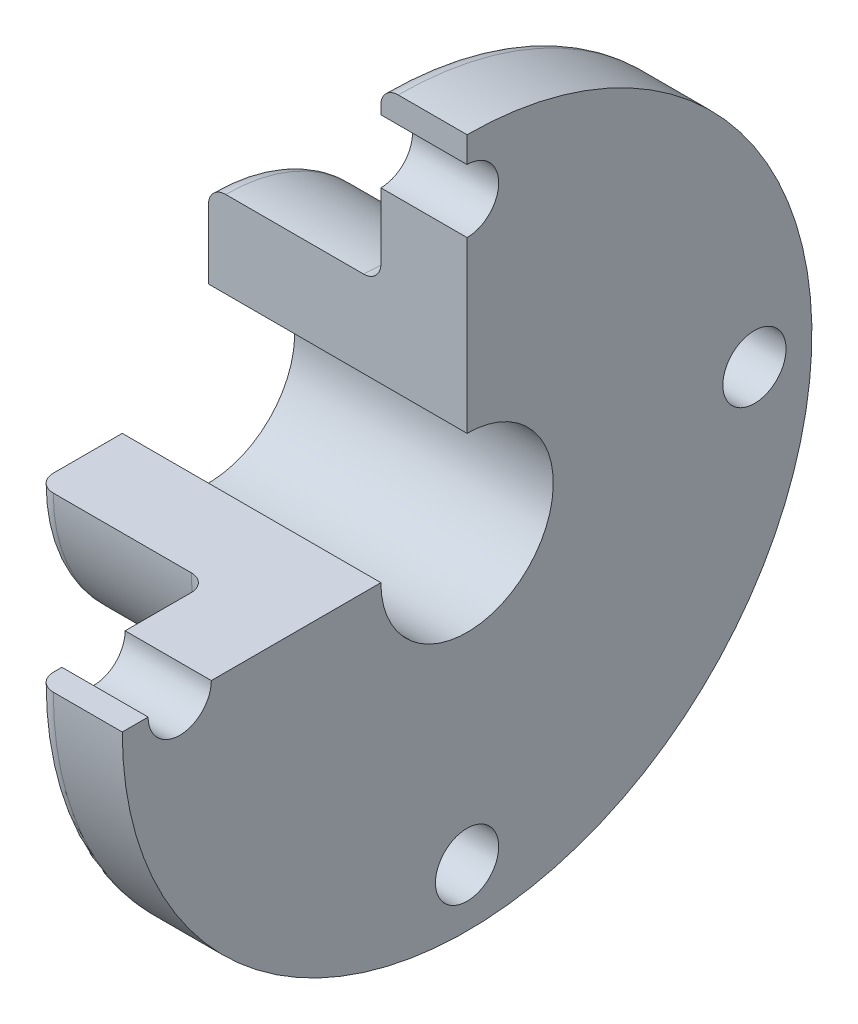
ISO-10303-21;
HEADER;
FILE_DESCRIPTION(('STEP AP214'),'2;1');
FILE_NAME('part.step','',(''),(''),'','','');
FILE_SCHEMA(('AUTOMOTIVE_DESIGN { 1 0 10303 214 1 1 1 1 }'));
ENDSEC;
DATA;
#1=APPLICATION_CONTEXT('core data for automotive mechanical design processes');
#2=APPLICATION_PROTOCOL_DEFINITION('international standard','automotive_design',2000,#1);
#3=PRODUCT_CONTEXT('',#1,'mechanical');
#4=PRODUCT('Part','Part','',(#3));
#5=PRODUCT_RELATED_PRODUCT_CATEGORY('part','',(#4));
#6=PRODUCT_DEFINITION_FORMATION('','',#4);
#7=PRODUCT_DEFINITION_CONTEXT('part definition',#1,'design');
#8=PRODUCT_DEFINITION('design','',#6,#7);
#9=PRODUCT_DEFINITION_SHAPE('','',#8);
#10=(LENGTH_UNIT() NAMED_UNIT(*) SI_UNIT(.MILLI.,.METRE.));
#11=(NAMED_UNIT(*) PLANE_ANGLE_UNIT() SI_UNIT($,.RADIAN.));
#12=(NAMED_UNIT(*) SI_UNIT($,.STERADIAN.) SOLID_ANGLE_UNIT());
#13=UNCERTAINTY_MEASURE_WITH_UNIT(LENGTH_MEASURE(1.E-05),#10,'distance_accuracy_value','');
#14=(GEOMETRIC_REPRESENTATION_CONTEXT(3) GLOBAL_UNCERTAINTY_ASSIGNED_CONTEXT((#13)) GLOBAL_UNIT_ASSIGNED_CONTEXT((#10,
#11,#12)) REPRESENTATION_CONTEXT('',''));
#15=CARTESIAN_POINT('',(0.,0.,0.));
#16=DIRECTION('',(0.,0.,1.));
#17=DIRECTION('',(1.,0.,0.));
#18=AXIS2_PLACEMENT_3D('',#15,#16,#17);
#19=CARTESIAN_POINT('',(17.9203539823009,0.,0.));
#20=DIRECTION('',(1.,0.,0.));
#21=DIRECTION('',(0.,0.,-1.));
#22=AXIS2_PLACEMENT_3D('',#19,#20,#21);
#23=PLANE('',#22);
#24=DIRECTION('',(0.,0.,1.));
#25=VECTOR('',#24,1.);
#26=CARTESIAN_POINT('',(17.9203539823009,0.,0.));
#27=LINE('',#26,#25);
#28=CARTESIAN_POINT('',(17.9203539823009,0.,55.5));
#29=VERTEX_POINT('',#28);
#30=CARTESIAN_POINT('',(17.9203539823009,0.,60.));
#31=VERTEX_POINT('',#30);
#32=EDGE_CURVE('E267',#29,#31,#27,.T.);
#33=ORIENTED_EDGE('',*,*,#32,.T.);
#34=CARTESIAN_POINT('',(17.9203539823009,0.,0.));
#35=DIRECTION('',(-1.,0.,0.));
#36=DIRECTION('',(0.,0.,1.));
#37=AXIS2_PLACEMENT_3D('',#34,#35,#36);
#38=CIRCLE('',#37,60.);
#39=CARTESIAN_POINT('',(17.9203539823009,60.,0.));
#40=VERTEX_POINT('',#39);
#41=EDGE_CURVE('E162',#40,#31,#38,.T.);
#42=ORIENTED_EDGE('',*,*,#41,.F.);
#43=DIRECTION('',(0.,-1.,0.));
#44=VECTOR('',#43,1.);
#45=CARTESIAN_POINT('',(17.9203539823009,77.9574634988186,0.));
#46=LINE('',#45,#44);
#47=CARTESIAN_POINT('',(17.9203539823009,55.5,0.));
#48=VERTEX_POINT('',#47);
#49=EDGE_CURVE('E272',#40,#48,#46,.T.);
#50=ORIENTED_EDGE('',*,*,#49,.T.);
#51=CARTESIAN_POINT('',(17.9203539823009,50.,0.));
#52=DIRECTION('',(-1.,0.,0.));
#53=DIRECTION('',(0.,0.,1.));
#54=AXIS2_PLACEMENT_3D('',#51,#52,#53);
#55=CIRCLE('',#54,5.5);
#56=CARTESIAN_POINT('',(17.9203539823009,44.5,0.));
#57=VERTEX_POINT('',#56);
#58=EDGE_CURVE('E229',#48,#57,#55,.T.);
#59=ORIENTED_EDGE('',*,*,#58,.T.);
#60=CARTESIAN_POINT('',(17.9203539823009,15.,0.));
#61=VERTEX_POINT('',#60);
#62=EDGE_CURVE('E270',#57,#61,#46,.T.);
#63=ORIENTED_EDGE('',*,*,#62,.T.);
#64=CARTESIAN_POINT('',(17.9203539823009,0.,0.));
#65=DIRECTION('',(-1.,0.,0.));
#66=DIRECTION('',(0.,0.,1.));
#67=AXIS2_PLACEMENT_3D('',#64,#65,#66);
#68=CIRCLE('',#67,15.);
#69=CARTESIAN_POINT('',(17.9203539823009,0.,15.));
#70=VERTEX_POINT('',#69);
#71=EDGE_CURVE('E231',#61,#70,#68,.T.);
#72=ORIENTED_EDGE('',*,*,#71,.T.);
#73=CARTESIAN_POINT('',(17.9203539823009,0.,44.5));
#74=VERTEX_POINT('',#73);
#75=EDGE_CURVE('E198',#70,#74,#27,.T.);
#76=ORIENTED_EDGE('',*,*,#75,.T.);
#77=CARTESIAN_POINT('',(17.9203539823009,-1.74574066942157E-13,50.));
#78=DIRECTION('',(-1.,0.,0.));
#79=DIRECTION('',(0.,0.,1.));
#80=AXIS2_PLACEMENT_3D('',#77,#78,#79);
#81=CIRCLE('',#80,5.5);
#82=EDGE_CURVE('E230',#74,#29,#81,.T.);
#83=ORIENTED_EDGE('',*,*,#82,.T.);
#84=EDGE_LOOP('',(#33,#42,#50,#59,#63,#72,#76,#83));
#85=FACE_BOUND('',#84,.T.);
#86=CARTESIAN_POINT('',(17.9203539823009,5.2372220082647E-13,-50.));
#87=DIRECTION('',(-1.,0.,0.));
#88=DIRECTION('',(0.,0.,1.));
#89=AXIS2_PLACEMENT_3D('',#86,#87,#88);
#90=CIRCLE('',#89,5.5);
#91=CARTESIAN_POINT('',(17.9203539823009,5.2372220082647E-13,-44.5));
#92=VERTEX_POINT('',#91);
#93=EDGE_CURVE('E238',#92,#92,#90,.T.);
#94=ORIENTED_EDGE('',*,*,#93,.T.);
#95=EDGE_LOOP('',(#94));
#96=FACE_BOUND('',#95,.T.);
#97=CARTESIAN_POINT('',(17.9203539823009,-50.,-3.49148133884313E-13));
#98=DIRECTION('',(-1.,0.,0.));
#99=DIRECTION('',(0.,0.,1.));
#100=AXIS2_PLACEMENT_3D('',#97,#98,#99);
#101=CIRCLE('',#100,5.5);
#102=CARTESIAN_POINT('',(17.9203539823009,-50.,5.49999999999965));
#103=VERTEX_POINT('',#102);
#104=EDGE_CURVE('E242',#103,#103,#101,.T.);
#105=ORIENTED_EDGE('',*,*,#104,.T.);
#106=EDGE_LOOP('',(#105));
#107=FACE_BOUND('',#106,.T.);
#108=ADVANCED_FACE('F43',(#85,#96,#107),#23,.T.);
#109=CARTESIAN_POINT('',(-55.7522123893804,0.,0.));
#110=DIRECTION('',(-1.,0.,0.));
#111=DIRECTION('',(0.,0.,1.));
#112=AXIS2_PLACEMENT_3D('',#109,#110,#111);
#113=CYLINDRICAL_SURFACE('',#112,60.);
#114=DIRECTION('',(-1.,0.,0.));
#115=VECTOR('',#114,1.);
#116=CARTESIAN_POINT('',(-55.7522123893804,0.,60.));
#117=LINE('',#116,#115);
#118=CARTESIAN_POINT('',(5.92035398230086,0.,60.));
#119=VERTEX_POINT('',#118);
#120=EDGE_CURVE('E204',#119,#31,#117,.F.);
#121=ORIENTED_EDGE('',*,*,#120,.F.);
#122=CARTESIAN_POINT('',(5.92035398230086,0.,0.));
#123=DIRECTION('',(-1.,0.,0.));
#124=DIRECTION('',(0.,0.,1.));
#125=AXIS2_PLACEMENT_3D('',#122,#123,#124);
#126=CIRCLE('',#125,60.);
#127=CARTESIAN_POINT('',(5.92035398230086,60.,0.));
#128=VERTEX_POINT('',#127);
#129=EDGE_CURVE('E178',#119,#128,#126,.F.);
#130=ORIENTED_EDGE('',*,*,#129,.T.);
#131=DIRECTION('',(-1.,0.,0.));
#132=VECTOR('',#131,1.);
#133=CARTESIAN_POINT('',(-55.7522123893804,60.,0.));
#134=LINE('',#133,#132);
#135=EDGE_CURVE('E190',#40,#128,#134,.T.);
#136=ORIENTED_EDGE('',*,*,#135,.F.);
#137=ORIENTED_EDGE('',*,*,#41,.T.);
#138=EDGE_LOOP('',(#121,#130,#136,#137));
#139=FACE_BOUND('',#138,.T.);
#140=ADVANCED_FACE('F209',(#139),#113,.T.);
#141=CARTESIAN_POINT('',(2.92035398230086,0.,0.));
#142=DIRECTION('',(-1.,0.,0.));
#143=DIRECTION('',(0.,0.,1.));
#144=AXIS2_PLACEMENT_3D('',#141,#142,#143);
#145=PLANE('',#144);
#146=DIRECTION('',(0.,0.,1.));
#147=VECTOR('',#146,1.);
#148=CARTESIAN_POINT('',(2.92035398230086,0.,0.));
#149=LINE('',#148,#147);
#150=CARTESIAN_POINT('',(2.92035398230086,0.,33.));
#151=VERTEX_POINT('',#150);
#152=CARTESIAN_POINT('',(2.92035398230086,0.,44.5));
#153=VERTEX_POINT('',#152);
#154=EDGE_CURVE('E217',#151,#153,#149,.T.);
#155=ORIENTED_EDGE('',*,*,#154,.F.);
#156=CARTESIAN_POINT('',(2.92035398230086,0.,0.));
#157=DIRECTION('',(-1.,0.,0.));
#158=DIRECTION('',(0.,0.,1.));
#159=AXIS2_PLACEMENT_3D('',#156,#157,#158);
#160=CIRCLE('',#159,33.);
#161=CARTESIAN_POINT('',(2.92035398230086,33.,0.));
#162=VERTEX_POINT('',#161);
#163=EDGE_CURVE('E174',#151,#162,#160,.F.);
#164=ORIENTED_EDGE('',*,*,#163,.T.);
#165=DIRECTION('',(0.,-1.,0.));
#166=VECTOR('',#165,1.);
#167=CARTESIAN_POINT('',(2.92035398230086,0.,0.));
#168=LINE('',#167,#166);
#169=CARTESIAN_POINT('',(2.92035398230086,44.5,0.));
#170=VERTEX_POINT('',#169);
#171=EDGE_CURVE('E66',#170,#162,#168,.T.);
#172=ORIENTED_EDGE('',*,*,#171,.F.);
#173=CARTESIAN_POINT('',(2.92035398230086,50.,0.));
#174=DIRECTION('',(-1.,0.,0.));
#175=DIRECTION('',(0.,0.,1.));
#176=AXIS2_PLACEMENT_3D('',#173,#174,#175);
#177=CIRCLE('',#176,5.5);
#178=CARTESIAN_POINT('',(2.92035398230086,55.5,0.));
#179=VERTEX_POINT('',#178);
#180=EDGE_CURVE('E197',#179,#170,#177,.T.);
#181=ORIENTED_EDGE('',*,*,#180,.F.);
#182=CARTESIAN_POINT('',(2.92035398230086,57.,0.));
#183=VERTEX_POINT('',#182);
#184=EDGE_CURVE('E183',#183,#179,#168,.T.);
#185=ORIENTED_EDGE('',*,*,#184,.F.);
#186=CARTESIAN_POINT('',(2.92035398230086,0.,0.));
#187=DIRECTION('',(-1.,0.,0.));
#188=DIRECTION('',(0.,0.,1.));
#189=AXIS2_PLACEMENT_3D('',#186,#187,#188);
#190=CIRCLE('',#189,57.);
#191=CARTESIAN_POINT('',(2.92035398230086,0.,57.));
#192=VERTEX_POINT('',#191);
#193=EDGE_CURVE('E175',#183,#192,#190,.T.);
#194=ORIENTED_EDGE('',*,*,#193,.T.);
#195=CARTESIAN_POINT('',(2.92035398230086,0.,55.5));
#196=VERTEX_POINT('',#195);
#197=EDGE_CURVE('E210',#196,#192,#149,.T.);
#198=ORIENTED_EDGE('',*,*,#197,.F.);
#199=CARTESIAN_POINT('',(2.92035398230086,-1.74574066942157E-13,50.));
#200=DIRECTION('',(-1.,0.,0.));
#201=DIRECTION('',(0.,0.,1.));
#202=AXIS2_PLACEMENT_3D('',#199,#200,#201);
#203=CIRCLE('',#202,5.5);
#204=EDGE_CURVE('E250',#153,#196,#203,.T.);
#205=ORIENTED_EDGE('',*,*,#204,.F.);
#206=EDGE_LOOP('',(#155,#164,#172,#181,#185,#194,#198,#205));
#207=FACE_BOUND('',#206,.T.);
#208=CARTESIAN_POINT('',(2.92035398230086,5.2372220082647E-13,-50.));
#209=DIRECTION('',(-1.,0.,0.));
#210=DIRECTION('',(0.,0.,1.));
#211=AXIS2_PLACEMENT_3D('',#208,#209,#210);
#212=CIRCLE('',#211,5.5);
#213=CARTESIAN_POINT('',(2.92035398230086,5.2372220082647E-13,-44.5));
#214=VERTEX_POINT('',#213);
#215=EDGE_CURVE('E232',#214,#214,#212,.T.);
#216=ORIENTED_EDGE('',*,*,#215,.F.);
#217=EDGE_LOOP('',(#216));
#218=FACE_BOUND('',#217,.T.);
#219=CARTESIAN_POINT('',(2.92035398230086,-50.,-3.49148133884313E-13));
#220=DIRECTION('',(-1.,0.,0.));
#221=DIRECTION('',(0.,0.,1.));
#222=AXIS2_PLACEMENT_3D('',#219,#220,#221);
#223=CIRCLE('',#222,5.5);
#224=CARTESIAN_POINT('',(2.92035398230086,-50.,5.49999999999965));
#225=VERTEX_POINT('',#224);
#226=EDGE_CURVE('E241',#225,#225,#223,.T.);
#227=ORIENTED_EDGE('',*,*,#226,.F.);
#228=EDGE_LOOP('',(#227));
#229=FACE_BOUND('',#228,.T.);
#230=ADVANCED_FACE('F191',(#207,#218,#229),#145,.T.);
#231=CARTESIAN_POINT('',(-55.7522123893804,0.,0.));
#232=DIRECTION('',(-1.,0.,0.));
#233=DIRECTION('',(0.,0.,1.));
#234=AXIS2_PLACEMENT_3D('',#231,#232,#233);
#235=CYLINDRICAL_SURFACE('',#234,30.);
#236=DIRECTION('',(-1.,0.,0.));
#237=VECTOR('',#236,1.);
#238=CARTESIAN_POINT('',(-55.7522123893804,0.,30.));
#239=LINE('',#238,#237);
#240=CARTESIAN_POINT('',(-24.0796460176991,0.,30.));
#241=VERTEX_POINT('',#240);
#242=CARTESIAN_POINT('',(-0.0796460176991434,0.,30.));
#243=VERTEX_POINT('',#242);
#244=EDGE_CURVE('E59',#241,#243,#239,.F.);
#245=ORIENTED_EDGE('',*,*,#244,.F.);
#246=CARTESIAN_POINT('',(-24.0796460176991,0.,0.));
#247=DIRECTION('',(-1.,0.,0.));
#248=DIRECTION('',(0.,0.,1.));
#249=AXIS2_PLACEMENT_3D('',#246,#247,#248);
#250=CIRCLE('',#249,30.);
#251=CARTESIAN_POINT('',(-24.0796460176991,30.,0.));
#252=VERTEX_POINT('',#251);
#253=EDGE_CURVE('E164',#241,#252,#250,.F.);
#254=ORIENTED_EDGE('',*,*,#253,.T.);
#255=DIRECTION('',(-1.,0.,0.));
#256=VECTOR('',#255,1.);
#257=CARTESIAN_POINT('',(-55.7522123893804,30.,0.));
#258=LINE('',#257,#256);
#259=CARTESIAN_POINT('',(-0.0796460176991434,30.,0.));
#260=VERTEX_POINT('',#259);
#261=EDGE_CURVE('E142',#260,#252,#258,.T.);
#262=ORIENTED_EDGE('',*,*,#261,.F.);
#263=CARTESIAN_POINT('',(-0.0796460176991434,0.,0.));
#264=DIRECTION('',(-1.,0.,0.));
#265=DIRECTION('',(0.,0.,1.));
#266=AXIS2_PLACEMENT_3D('',#263,#264,#265);
#267=CIRCLE('',#266,30.);
#268=EDGE_CURVE('E163',#260,#243,#267,.T.);
#269=ORIENTED_EDGE('',*,*,#268,.T.);
#270=EDGE_LOOP('',(#245,#254,#262,#269));
#271=FACE_BOUND('',#270,.T.);
#272=ADVANCED_FACE('F283',(#271),#235,.T.);
#273=CARTESIAN_POINT('',(-27.0796460176991,0.,0.));
#274=DIRECTION('',(-1.,0.,0.));
#275=DIRECTION('',(0.,0.,1.));
#276=AXIS2_PLACEMENT_3D('',#273,#274,#275);
#277=PLANE('',#276);
#278=DIRECTION('',(0.,0.,1.));
#279=VECTOR('',#278,1.);
#280=CARTESIAN_POINT('',(-27.0796460176991,0.,0.));
#281=LINE('',#280,#279);
#282=CARTESIAN_POINT('',(-27.0796460176991,0.,15.));
#283=VERTEX_POINT('',#282);
#284=CARTESIAN_POINT('',(-27.0796460176991,0.,27.));
#285=VERTEX_POINT('',#284);
#286=EDGE_CURVE('E156',#283,#285,#281,.T.);
#287=ORIENTED_EDGE('',*,*,#286,.F.);
#288=CARTESIAN_POINT('',(-27.0796460176991,0.,0.));
#289=DIRECTION('',(-1.,0.,0.));
#290=DIRECTION('',(0.,0.,1.));
#291=AXIS2_PLACEMENT_3D('',#288,#289,#290);
#292=CIRCLE('',#291,15.);
#293=CARTESIAN_POINT('',(-27.0796460176991,15.,0.));
#294=VERTEX_POINT('',#293);
#295=EDGE_CURVE('E154',#294,#283,#292,.T.);
#296=ORIENTED_EDGE('',*,*,#295,.F.);
#297=DIRECTION('',(0.,-1.,0.));
#298=VECTOR('',#297,1.);
#299=CARTESIAN_POINT('',(-27.0796460176991,77.9574634988186,0.));
#300=LINE('',#299,#298);
#301=CARTESIAN_POINT('',(-27.0796460176991,27.,0.));
#302=VERTEX_POINT('',#301);
#303=EDGE_CURVE('E138',#302,#294,#300,.T.);
#304=ORIENTED_EDGE('',*,*,#303,.F.);
#305=CARTESIAN_POINT('',(-27.0796460176991,0.,0.));
#306=DIRECTION('',(-1.,0.,0.));
#307=DIRECTION('',(0.,0.,1.));
#308=AXIS2_PLACEMENT_3D('',#305,#306,#307);
#309=CIRCLE('',#308,27.);
#310=EDGE_CURVE('E152',#302,#285,#309,.T.);
#311=ORIENTED_EDGE('',*,*,#310,.T.);
#312=EDGE_LOOP('',(#287,#296,#304,#311));
#313=FACE_BOUND('',#312,.T.);
#314=ADVANCED_FACE('F155',(#313),#277,.T.);
#315=CARTESIAN_POINT('',(-55.7522123893804,0.,0.));
#316=DIRECTION('',(-1.,0.,0.));
#317=DIRECTION('',(0.,0.,1.));
#318=AXIS2_PLACEMENT_3D('',#315,#316,#317);
#319=CYLINDRICAL_SURFACE('',#318,15.);
#320=DIRECTION('',(-1.,0.,0.));
#321=VECTOR('',#320,1.);
#322=CARTESIAN_POINT('',(-55.7522123893804,0.,15.));
#323=LINE('',#322,#321);
#324=EDGE_CURVE('E227',#70,#283,#323,.T.);
#325=ORIENTED_EDGE('',*,*,#324,.F.);
#326=ORIENTED_EDGE('',*,*,#71,.F.);
#327=DIRECTION('',(-1.,0.,0.));
#328=VECTOR('',#327,1.);
#329=CARTESIAN_POINT('',(-55.7522123893804,15.,0.));
#330=LINE('',#329,#328);
#331=EDGE_CURVE('E216',#294,#61,#330,.F.);
#332=ORIENTED_EDGE('',*,*,#331,.F.);
#333=ORIENTED_EDGE('',*,*,#295,.T.);
#334=EDGE_LOOP('',(#325,#326,#332,#333));
#335=FACE_BOUND('',#334,.T.);
#336=ADVANCED_FACE('F253',(#335),#319,.F.);
#337=CARTESIAN_POINT('',(17.9203539823009,-1.74574066942157E-13,50.));
#338=DIRECTION('',(-1.,0.,0.));
#339=DIRECTION('',(0.,0.,1.));
#340=AXIS2_PLACEMENT_3D('',#337,#338,#339);
#341=CYLINDRICAL_SURFACE('',#340,5.5);
#342=ORIENTED_EDGE('',*,*,#204,.T.);
#343=DIRECTION('',(-1.,0.,0.));
#344=VECTOR('',#343,1.);
#345=CARTESIAN_POINT('',(17.9203539823009,0.,55.5));
#346=LINE('',#345,#344);
#347=EDGE_CURVE('E212',#196,#29,#346,.F.);
#348=ORIENTED_EDGE('',*,*,#347,.T.);
#349=ORIENTED_EDGE('',*,*,#82,.F.);
#350=DIRECTION('',(-1.,0.,0.));
#351=VECTOR('',#350,1.);
#352=CARTESIAN_POINT('',(17.9203539823009,0.,44.5));
#353=LINE('',#352,#351);
#354=EDGE_CURVE('E222',#74,#153,#353,.T.);
#355=ORIENTED_EDGE('',*,*,#354,.T.);
#356=EDGE_LOOP('',(#342,#348,#349,#355));
#357=FACE_BOUND('',#356,.T.);
#358=ADVANCED_FACE('F323',(#357),#341,.F.);
#359=CARTESIAN_POINT('',(17.9203539823009,-50.,-3.49148133884313E-13));
#360=DIRECTION('',(-1.,0.,0.));
#361=DIRECTION('',(0.,0.,1.));
#362=AXIS2_PLACEMENT_3D('',#359,#360,#361);
#363=CYLINDRICAL_SURFACE('',#362,5.5);
#364=ORIENTED_EDGE('',*,*,#104,.F.);
#365=EDGE_LOOP('',(#364));
#366=FACE_BOUND('',#365,.T.);
#367=ORIENTED_EDGE('',*,*,#226,.T.);
#368=EDGE_LOOP('',(#367));
#369=FACE_BOUND('',#368,.T.);
#370=ADVANCED_FACE('F330',(#366,#369),#363,.F.);
#371=CARTESIAN_POINT('',(17.9203539823009,5.2372220082647E-13,-50.));
#372=DIRECTION('',(-1.,0.,0.));
#373=DIRECTION('',(0.,0.,1.));
#374=AXIS2_PLACEMENT_3D('',#371,#372,#373);
#375=CYLINDRICAL_SURFACE('',#374,5.5);
#376=ORIENTED_EDGE('',*,*,#93,.F.);
#377=EDGE_LOOP('',(#376));
#378=FACE_BOUND('',#377,.T.);
#379=ORIENTED_EDGE('',*,*,#215,.T.);
#380=EDGE_LOOP('',(#379));
#381=FACE_BOUND('',#380,.T.);
#382=ADVANCED_FACE('F332',(#378,#381),#375,.F.);
#383=CARTESIAN_POINT('',(17.9203539823009,50.,0.));
#384=DIRECTION('',(-1.,0.,0.));
#385=DIRECTION('',(0.,0.,1.));
#386=AXIS2_PLACEMENT_3D('',#383,#384,#385);
#387=CYLINDRICAL_SURFACE('',#386,5.5);
#388=ORIENTED_EDGE('',*,*,#180,.T.);
#389=DIRECTION('',(-1.,0.,0.));
#390=VECTOR('',#389,1.);
#391=CARTESIAN_POINT('',(17.9203539823009,44.5,0.));
#392=LINE('',#391,#390);
#393=EDGE_CURVE('E147',#170,#57,#392,.F.);
#394=ORIENTED_EDGE('',*,*,#393,.T.);
#395=ORIENTED_EDGE('',*,*,#58,.F.);
#396=DIRECTION('',(-1.,0.,0.));
#397=VECTOR('',#396,1.);
#398=CARTESIAN_POINT('',(17.9203539823009,55.5,0.));
#399=LINE('',#398,#397);
#400=EDGE_CURVE('E263',#48,#179,#399,.T.);
#401=ORIENTED_EDGE('',*,*,#400,.T.);
#402=EDGE_LOOP('',(#388,#394,#395,#401));
#403=FACE_BOUND('',#402,.T.);
#404=ADVANCED_FACE('F280',(#403),#387,.F.);
#405=CARTESIAN_POINT('',(-24.0796460176991,0.,0.));
#406=DIRECTION('',(-1.,0.,0.));
#407=DIRECTION('',(0.,0.,1.));
#408=AXIS2_PLACEMENT_3D('',#405,#406,#407);
#409=TOROIDAL_SURFACE('',#408,27.,3.);
#410=CARTESIAN_POINT('',(-24.0796460176991,0.,27.));
#411=DIRECTION('',(0.,-1.,0.));
#412=DIRECTION('',(0.,0.,-1.));
#413=AXIS2_PLACEMENT_3D('',#410,#411,#412);
#414=CIRCLE('',#413,3.);
#415=EDGE_CURVE('E159',#285,#241,#414,.F.);
#416=ORIENTED_EDGE('',*,*,#415,.F.);
#417=ORIENTED_EDGE('',*,*,#310,.F.);
#418=CARTESIAN_POINT('',(-24.0796460176991,27.,0.));
#419=DIRECTION('',(0.,0.,-1.));
#420=DIRECTION('',(-1.,0.,0.));
#421=AXIS2_PLACEMENT_3D('',#418,#419,#420);
#422=CIRCLE('',#421,3.);
#423=EDGE_CURVE('E134',#252,#302,#422,.F.);
#424=ORIENTED_EDGE('',*,*,#423,.F.);
#425=ORIENTED_EDGE('',*,*,#253,.F.);
#426=EDGE_LOOP('',(#416,#417,#424,#425));
#427=FACE_BOUND('',#426,.T.);
#428=ADVANCED_FACE('F157',(#427),#409,.T.);
#429=CARTESIAN_POINT('',(-0.0796460176991434,0.,0.));
#430=DIRECTION('',(-1.,0.,0.));
#431=DIRECTION('',(0.,0.,1.));
#432=AXIS2_PLACEMENT_3D('',#429,#430,#431);
#433=TOROIDAL_SURFACE('',#432,33.,3.);
#434=ORIENTED_EDGE('',*,*,#163,.F.);
#435=CARTESIAN_POINT('',(-0.0796460176991434,0.,33.));
#436=DIRECTION('',(0.,-1.,0.));
#437=DIRECTION('',(0.,0.,-1.));
#438=AXIS2_PLACEMENT_3D('',#435,#436,#437);
#439=CIRCLE('',#438,3.);
#440=EDGE_CURVE('E211',#151,#243,#439,.F.);
#441=ORIENTED_EDGE('',*,*,#440,.T.);
#442=ORIENTED_EDGE('',*,*,#268,.F.);
#443=CARTESIAN_POINT('',(-0.0796460176991434,33.,0.));
#444=DIRECTION('',(0.,0.,-1.));
#445=DIRECTION('',(-1.,0.,0.));
#446=AXIS2_PLACEMENT_3D('',#443,#444,#445);
#447=CIRCLE('',#446,3.);
#448=EDGE_CURVE('E265',#260,#162,#447,.F.);
#449=ORIENTED_EDGE('',*,*,#448,.T.);
#450=EDGE_LOOP('',(#434,#441,#442,#449));
#451=FACE_BOUND('',#450,.T.);
#452=ADVANCED_FACE('F281',(#451),#433,.F.);
#453=CARTESIAN_POINT('',(5.92035398230086,0.,0.));
#454=DIRECTION('',(-1.,0.,0.));
#455=DIRECTION('',(0.,0.,1.));
#456=AXIS2_PLACEMENT_3D('',#453,#454,#455);
#457=TOROIDAL_SURFACE('',#456,57.,3.);
#458=CARTESIAN_POINT('',(5.92035398230086,0.,57.));
#459=DIRECTION('',(0.,-1.,0.));
#460=DIRECTION('',(0.,0.,-1.));
#461=AXIS2_PLACEMENT_3D('',#458,#459,#460);
#462=CIRCLE('',#461,3.);
#463=EDGE_CURVE('E11',#192,#119,#462,.F.);
#464=ORIENTED_EDGE('',*,*,#463,.F.);
#465=ORIENTED_EDGE('',*,*,#193,.F.);
#466=CARTESIAN_POINT('',(5.92035398230086,57.,0.));
#467=DIRECTION('',(0.,0.,-1.));
#468=DIRECTION('',(-1.,0.,0.));
#469=AXIS2_PLACEMENT_3D('',#466,#467,#468);
#470=CIRCLE('',#469,3.);
#471=EDGE_CURVE('E51',#128,#183,#470,.F.);
#472=ORIENTED_EDGE('',*,*,#471,.F.);
#473=ORIENTED_EDGE('',*,*,#129,.F.);
#474=EDGE_LOOP('',(#464,#465,#472,#473));
#475=FACE_BOUND('',#474,.T.);
#476=ADVANCED_FACE('F44',(#475),#457,.T.);
#477=CARTESIAN_POINT('',(17.9203539823009,77.9574634988186,0.));
#478=DIRECTION('',(0.,0.,-1.));
#479=DIRECTION('',(-1.,0.,0.));
#480=AXIS2_PLACEMENT_3D('',#477,#478,#479);
#481=PLANE('',#480);
#482=ORIENTED_EDGE('',*,*,#49,.F.);
#483=ORIENTED_EDGE('',*,*,#135,.T.);
#484=ORIENTED_EDGE('',*,*,#471,.T.);
#485=ORIENTED_EDGE('',*,*,#184,.T.);
#486=ORIENTED_EDGE('',*,*,#400,.F.);
#487=EDGE_LOOP('',(#482,#483,#484,#485,#486));
#488=FACE_BOUND('',#487,.T.);
#489=ADVANCED_FACE('F182',(#488),#481,.F.);
#490=CARTESIAN_POINT('',(17.9203539823009,0.,0.));
#491=DIRECTION('',(0.,-1.,0.));
#492=DIRECTION('',(0.,0.,-1.));
#493=AXIS2_PLACEMENT_3D('',#490,#491,#492);
#494=PLANE('',#493);
#495=ORIENTED_EDGE('',*,*,#197,.T.);
#496=ORIENTED_EDGE('',*,*,#463,.T.);
#497=ORIENTED_EDGE('',*,*,#120,.T.);
#498=ORIENTED_EDGE('',*,*,#32,.F.);
#499=ORIENTED_EDGE('',*,*,#347,.F.);
#500=EDGE_LOOP('',(#495,#496,#497,#498,#499));
#501=FACE_BOUND('',#500,.T.);
#502=ADVANCED_FACE('F202',(#501),#494,.F.);
#503=ORIENTED_EDGE('',*,*,#331,.T.);
#504=ORIENTED_EDGE('',*,*,#62,.F.);
#505=ORIENTED_EDGE('',*,*,#393,.F.);
#506=ORIENTED_EDGE('',*,*,#171,.T.);
#507=ORIENTED_EDGE('',*,*,#448,.F.);
#508=ORIENTED_EDGE('',*,*,#261,.T.);
#509=ORIENTED_EDGE('',*,*,#423,.T.);
#510=ORIENTED_EDGE('',*,*,#303,.T.);
#511=EDGE_LOOP('',(#503,#504,#505,#506,#507,#508,#509,#510));
#512=FACE_BOUND('',#511,.T.);
#513=ADVANCED_FACE('F140',(#512),#481,.F.);
#514=ORIENTED_EDGE('',*,*,#324,.T.);
#515=ORIENTED_EDGE('',*,*,#286,.T.);
#516=ORIENTED_EDGE('',*,*,#415,.T.);
#517=ORIENTED_EDGE('',*,*,#244,.T.);
#518=ORIENTED_EDGE('',*,*,#440,.F.);
#519=ORIENTED_EDGE('',*,*,#154,.T.);
#520=ORIENTED_EDGE('',*,*,#354,.F.);
#521=ORIENTED_EDGE('',*,*,#75,.F.);
#522=EDGE_LOOP('',(#514,#515,#516,#517,#518,#519,#520,#521));
#523=FACE_BOUND('',#522,.T.);
#524=ADVANCED_FACE('F313',(#523),#494,.F.);
#525=CLOSED_SHELL('',(#108,#140,#230,#272,#314,#336,#358,#370,#382,#404,#428,#452,#476,#489,
#502,#513,#524));
#526=MANIFOLD_SOLID_BREP('B2',#525);
#527=ADVANCED_BREP_SHAPE_REPRESENTATION('',(#18,#526),#14);
#528=SHAPE_DEFINITION_REPRESENTATION(#9,#527);
ENDSEC;
END-ISO-10303-21;
